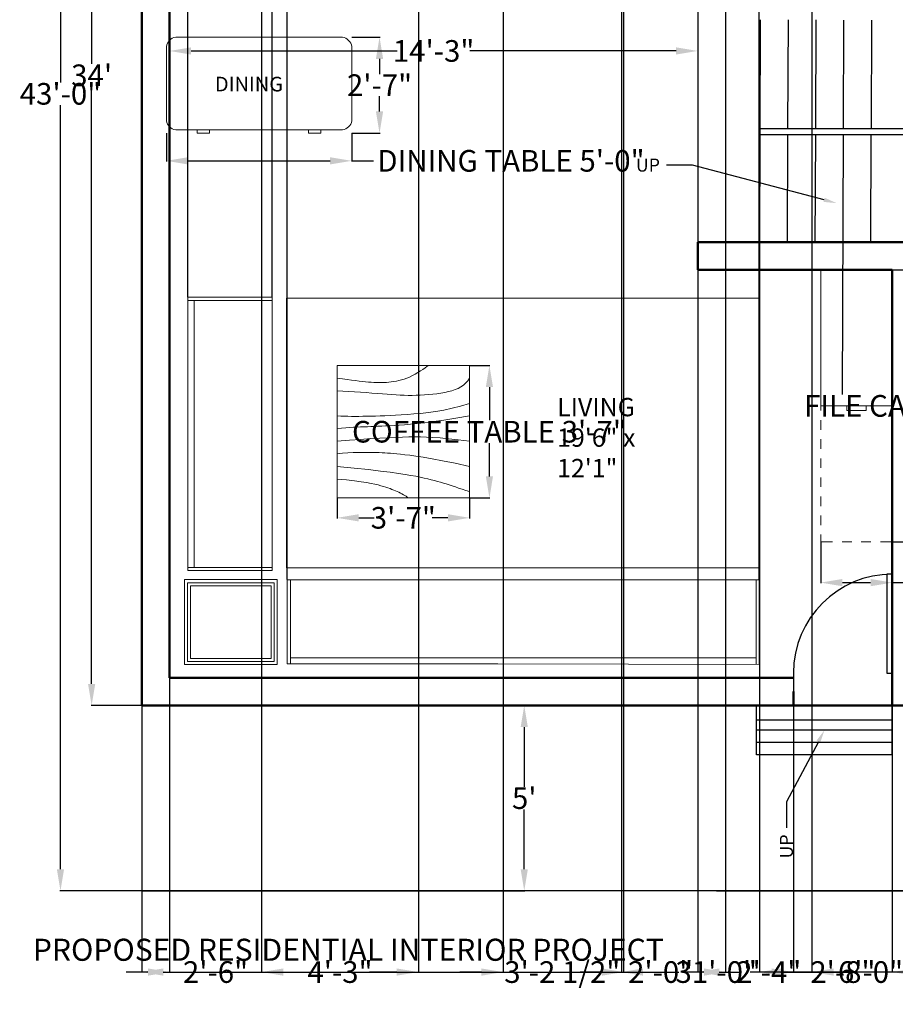
# Model space of a CAD drawing. Units: inches. Extents: x 164 to 612, y 17 to 606.
# Tile 1 of 3: x 164 to 448, y 17 to 335. Entities that reach past the tile are written whole.
import ezdxf
from ezdxf import colors
from ezdxf.entities.mleader import LeaderData, LeaderLine
from ezdxf.math import Vec2, Vec3

# ---------------------------------------------------------------- set-up
doc = ezdxf.new("R2010")
doc.units = ezdxf.units.IN
doc.header["$MEASUREMENT"] = 0
for name, color, linetype, lineweight in [('A-ANNO-DIMS', 2, 'Continuous', 18), ('A-ANNO-TEXT', 7, 'Continuous', 18), ('A-ANNO-TTLB', 7, 'Continuous', 35), ('A-AREA-IDEN', 7, 'Continuous', 25), ('A-DOOR', 4, 'Continuous', 25), ('A-FLOR-STRS', 7, 'Continuous', 25), ('A-FURN', 8, 'Continuous', 18), ('A-WALL', 7, 'Continuous', 50), ('C-PROP', 3, 'Continuous', 25)]:
    doc.layers.add(name, color=color, linetype=linetype, lineweight=lineweight)
doc.styles.get("Standard").update_dxf_attribs({"font": 'arial.ttf'})
doc.dimstyles.get("Standard").update_dxf_attribs({"dimtxt": 7, "dimasz": 7, "dimexe": 0.18, "dimexo": 0.0625, "dimgap": 0.09, "dimtad": 0, "dimtih": 1, "dimtoh": 1, "dimdec": 0, "dimzin": 0, "dimdsep": 46, "dimlunit": 3, "dimtxsty": 'Standard', "dimcen": 0.09, "dimadec": 0, "dimazin": 0, "dimtfac": 1, "dimtdec": 0, "dimtofl": 0, "dimtmove": 0, "dimatfit": 3, "dimfxl": 1, "dimtolj": 1, "dimtzin": 0, "dimarcsym": 0})

# ---------------------------------------------------------------- blocks, each defined once
blk = doc.blocks.new('File Cabinet - Letter')
for p, q in [((0, 0), (15, 0)), ((0, -28.5), (0, 0)), ((15, 0), (15, -28.5)), ((15, -28.5), (0, -28.5)), ((0, -29.5), (0, -28.5)), ((5.5, -28.5), (5.5, -29.5)), ((9.5, -29.5), (9.5, -28.5)), ((5.5, -29.5), (9.5, -29.5)), ((15, -30.5), (15, -32.5)), ((0, -33.5), (0, -31.5)), ((15, -34.5), (15, -36.5)), ((0, -37.5), (0, -35.5)), ((15, -38.5), (15, -40.5)), ((0, -41.5), (0, -39.5)), ((15, -42.5), (15, -44.5)), ((0, -45.5), (0, -43.5)), ((15, -46.5), (15, -48.5)), ((0, -49.5), (0, -47.5)), ((0, -53.5), (0, -51.5)), ((15, -50.5), (15, -52.5)), ((0, -57), (0, -55.5)), ((15, -54.5), (15, -57)), ((2.5, -57), (0, -57)), ((6.5, -57), (4.5, -57)), ((10.5, -57), (8.5, -57)), ((15, -57), (12.5, -57))]:
    blk.add_line(p, q)
blk = doc.blocks.new('Table - Square Woodgrain 42 x 42 in.')
blk.add_line((0, -42), (42, -42))
for points in [[(0, -4), (1.704, -4.2172), (3.2358, -4.4188), (4.615, -4.604), (5.8615, -4.7721), (6.9951, -4.9224), (8.0357, -5.0541), (9.0031, -5.1667), (9.9171, -5.2594), (10.7951, -5.3316), (11.6445, -5.3836), (12.4702, -5.4157), (13.277, -5.4283), (14.0698, -5.4217), (14.8535, -5.3964), (15.6331, -5.3526), (16.4133, -5.2908), (17.1986, -5.2103), (17.9913, -5.1062), (18.793, -4.9727), (19.6056, -4.8038), (20.4307, -4.5937), (21.2701, -4.3365), (22.1256, -4.0262), (22.9989, -3.6571), (23.888, -3.2272), (24.7756, -2.7516), (25.6408, -2.2491), (26.4624, -1.7387), (27.2195, -1.2395), (27.891, -0.7703), (28.456, -0.3501), (28.8934, 0.002)], [(0, -42), (0, 0), (42, 0), (42, -42)], [(0, -8), (1.8203, -8.1001), (3.6741, -8.2149), (5.5411, -8.3408), (7.4011, -8.4741), (9.2339, -8.6112), (11.0193, -8.7484), (12.7371, -8.8821), (14.3671, -9.0086), (15.8954, -9.1246), (17.3337, -9.2278), (18.6997, -9.3159), (20.0116, -9.387), (21.2871, -9.4389), (22.5442, -9.4696), (23.8008, -9.477), (25.0749, -9.459), (26.3791, -9.4137), (27.7049, -9.3403), (29.0383, -9.2382), (30.3655, -9.1068), (31.6728, -8.9455), (32.9461, -8.7535), (34.1717, -8.5304), (35.3358, -8.2756), (36.4268, -7.9863), (37.443, -7.6521), (38.3849, -7.2603), (39.253, -6.7986), (40.048, -6.2542), (40.7705, -5.6147), (41.421, -4.8674), (42, -4)], [(42, -12), (39.1784, -12.8621), (36.4519, -13.5654), (33.8246, -14.1294), (31.3004, -14.5731), (28.8832, -14.9161), (26.577, -15.1775), (24.3858, -15.3768), (22.3136, -15.5332), (20.3622, -15.6632), (18.5254, -15.7718), (16.7947, -15.8612), (15.1618, -15.9338), (13.6183, -15.9916), (12.1558, -16.0369), (10.7659, -16.0718), (9.4403, -16.0987), (8.1703, -16.1191), (6.9461, -16.1325), (5.7577, -16.1377), (4.595, -16.1335), (3.4479, -16.1188), (2.3064, -16.0924), (1.1604, -16.0532), (0, -16)], [(42, -16), (37.6529, -16.7365), (33.8802, -17.329), (30.6179, -17.7961), (27.8015, -18.1561), (25.3668, -18.4275), (23.2497, -18.6288), (21.3859, -18.7785), (19.7111, -18.8949), (18.1693, -18.9939), (16.7375, -19.0795), (15.401, -19.1534), (14.1449, -19.217), (12.9544, -19.2717), (11.8148, -19.3191), (10.7113, -19.3606), (9.6291, -19.3976), (8.5534, -19.4323), (7.47, -19.4689), (6.3643, -19.5122), (5.222, -19.5672), (4.0288, -19.6386), (2.7703, -19.7313), (1.4321, -19.8501), (0, -20)], [(0, -24), (3.9243, -23.6805), (7.4766, -23.4138), (10.6891, -23.1954), (13.5943, -23.0205), (16.2247, -22.8847), (18.6125, -22.7832), (20.7903, -22.7116), (22.7903, -22.6651), (24.6563, -22.642), (26.4764, -22.6507), (28.35, -22.7024), (30.3766, -22.8084), (32.6555, -22.98), (35.2861, -23.2283), (38.3678, -23.5645), (42, -24)], [(42, -32), (37.392, -31.017), (33.4585, -30.2231), (30.1291, -29.5949), (27.3334, -29.109), (25.0009, -28.742), (23.0612, -28.4707), (21.4439, -28.2716), (20.0786, -28.1215), (18.8998, -28.0002), (17.8609, -27.9014), (16.9206, -27.8219), (16.0371, -27.7588), (15.1691, -27.709), (14.2748, -27.6693), (13.3128, -27.6368), (12.2415, -27.6083), (11.0295, -27.5824), (9.6867, -27.5643), (8.233, -27.5608), (6.6884, -27.5787), (5.0728, -27.6248), (3.4062, -27.7058), (1.7086, -27.8286), (0, -28)], [(0, -32), (5.4026, -32.5358), (9.9494, -33.019), (13.7424, -33.4553), (16.8834, -33.8505), (19.4743, -34.2106), (21.6171, -34.5413), (23.4136, -34.8486), (24.9657, -35.1382), (26.3614, -35.4156), (27.6332, -35.6841), (28.7995, -35.9467), (29.8788, -36.2064), (30.8897, -36.4661), (31.8507, -36.7288), (32.7802, -36.9973), (33.6968, -37.2747), (34.6175, -37.5635), (35.5531, -37.8651), (36.5128, -38.1805), (37.506, -38.5108), (38.5421, -38.8568), (39.6302, -39.2197), (40.7797, -39.6004), (42, -40)], [(0, -36), (3.0098, -36.2857), (5.5354, -36.5643), (7.6368, -36.8359), (9.374, -37.1009), (10.807, -37.3597), (11.9957, -37.6126), (13.0002, -37.8599), (13.8804, -38.102), (14.6874, -38.3393), (15.4365, -38.5729), (16.1338, -38.8041), (16.7858, -39.0341), (17.3987, -39.264), (17.9787, -39.4952), (18.5322, -39.7288), (19.0655, -39.9662), (19.5832, -40.2081), (20.0842, -40.4544), (20.5657, -40.7046), (21.0249, -40.9581), (21.459, -41.2144), (21.8653, -41.4731), (22.2409, -41.7335), (22.5831, -41.9951)]]:
    blk.add_lwpolyline(points)
blk = doc.blocks.new('Desk - 30 x 60 in.')
for p, q in [((-26.999995, 0), (26.999995, 0)), ((-29.999995, -27), (-29.999995, -3)), ((29.999995, -3), (29.999995, -27)), ((26.999995, -30), (-26.999995, -30)), ((-20.000005, -30), (-20.000005, -31)), ((-20.000005, -31), (-16.000005, -31)), ((-16.000005, -31), (-16.000005, -30)), ((15.999995, -31), (15.999995, -30)), ((19.999995, -31), (15.999995, -31)), ((19.999995, -30), (19.999995, -31))]:
    blk.add_line(p, q)
for centre, start, end in [((-26.499995, -3.5), 98.1301, 171.8699), ((26.499995, -3.5), 8.130102, 81.8699), ((-26.499995, -26.5), 188.1301, 261.8699), ((26.499995, -26.5), 278.1301, 351.8699)]:
    blk.add_arc(centre, 3.535534, start, end)
blk = doc.blocks.new('*U11')
for p, q in [((0, 0), (0, -6)), ((-32, 0), (-32, -6))]:
    blk.add_line(p, q)
blk.add_lwpolyline([(0, 0), (0, 32), (-1.75, 32), (-1.75, 0)], close=True)
blk.add_arc((0, 0), 32, 90, 180)
blk = doc.blocks.new('*D17')
at = {"layer": 'A-ANNO-DIMS', "color": 0, "lineweight": -2, "transparency": 16777216}
for p, q in [((481.01, 254.38), (468.54, 254.38)), ((468.72, 247.38), (468.72, 157.54)), ((468.72, 60.38), (468.72, 150.22)), ((389.63, 53.38), (468.9, 53.38))]:
    blk.add_line(p, q, dxfattribs=at)
at = {"layer": 'A-ANNO-DIMS', "color": 0, "transparency": 16777216}
for points in [[(467.56, 247.38), (469.89, 247.38), (468.72, 254.38)], [(467.56, 60.38), (469.89, 60.38), (468.72, 53.38)]]:
    blk.add_solid(points, dxfattribs=at)
at = {"layer": 'Defpoints', "color": 0, "transparency": 16777216}
for p in [(481.07, 254.38), (389.57, 53.38), (468.72, 53.38)]:
    blk.add_point(p, dxfattribs=at)
at = {"layer": 'A-ANNO-DIMS', "color": 0, "transparency": 16777216, "insert": (468.72, 153.88), "char_height": 7, "attachment_point": 5}
blk.add_mtext('\\A1;16\'-9"', dxfattribs=at)
blk = doc.blocks.new('*D18')
at = {"layer": 'A-ANNO-DIMS', "color": 0, "lineweight": -2, "transparency": 16777216}
for p, q in [((203.63, 113.38), (327.6, 113.38)), ((327.42, 106.38), (327.42, 87.03)), ((327.42, 60.38), (327.42, 79.73)), ((203.63, 53.38), (327.6, 53.38))]:
    blk.add_line(p, q, dxfattribs=at)
at = {"layer": 'A-ANNO-DIMS', "color": 0, "transparency": 16777216}
for points in [[(326.25, 106.38), (328.59, 106.38), (327.42, 113.38)], [(326.25, 60.38), (328.59, 60.38), (327.42, 53.38)]]:
    blk.add_solid(points, dxfattribs=at)
at = {"layer": 'Defpoints', "color": 0, "transparency": 16777216}
for p in [(203.57, 113.38), (203.57, 53.38), (327.42, 53.38)]:
    blk.add_point(p, dxfattribs=at)
at = {"layer": 'A-ANNO-DIMS', "color": 0, "transparency": 16777216, "insert": (327.42, 83.38), "char_height": 7, "attachment_point": 5}
blk.add_mtext("\\A1;5'", dxfattribs=at)
blk = doc.blocks.new('*D20')
at = {"layer": 'A-ANNO-DIMS', "color": 0, "lineweight": -2, "transparency": 16777216}
for p, q in [((212.57, 401.32), (212.57, 325.08)), ((383.57, 335.32), (383.57, 325.08)), ((219.57, 325.26), (286.29, 325.26)), ((376.57, 325.26), (309.85, 325.26))]:
    blk.add_line(p, q, dxfattribs=at)
at = {"layer": 'A-ANNO-DIMS', "color": 0, "transparency": 16777216}
for points in [[(219.57, 326.42), (219.57, 324.09), (212.57, 325.26)], [(376.57, 326.42), (376.57, 324.09), (383.57, 325.26)]]:
    blk.add_solid(points, dxfattribs=at)
at = {"layer": 'Defpoints', "color": 0, "transparency": 16777216}
for p in [(212.57, 401.38), (383.57, 335.38), (212.57, 325.26)]:
    blk.add_point(p, dxfattribs=at)
at = {"layer": 'A-ANNO-DIMS', "color": 0, "transparency": 16777216, "insert": (298.07, 325.26), "char_height": 7, "attachment_point": 5}
blk.add_mtext('\\A1;14\'-3"', dxfattribs=at)
blk = doc.blocks.new('*D21')
at = {"layer": 'A-ANNO-DIMS', "color": 0, "lineweight": -2, "transparency": 16777216}
for p, q in [((227.33, 521.38), (187.19, 521.38)), ((187.37, 514.38), (187.37, 321.05)), ((187.37, 120.38), (187.37, 313.71)), ((217.32, 113.38), (187.19, 113.38))]:
    blk.add_line(p, q, dxfattribs=at)
at = {"layer": 'A-ANNO-DIMS', "color": 0, "transparency": 16777216}
for points in [[(186.2, 514.38), (188.54, 514.38), (187.37, 521.38)], [(186.2, 120.38), (188.54, 120.38), (187.37, 113.38)]]:
    blk.add_solid(points, dxfattribs=at)
at = {"layer": 'Defpoints', "color": 0, "transparency": 16777216}
for p in [(227.39, 521.38), (187.37, 113.38), (217.38, 113.38)]:
    blk.add_point(p, dxfattribs=at)
at = {"layer": 'A-ANNO-DIMS', "color": 0, "transparency": 16777216, "insert": (187.37, 317.38), "char_height": 7, "attachment_point": 5}
blk.add_mtext("\\A1;34'", dxfattribs=at)
blk = doc.blocks.new('*D30')
at = {"layer": 'A-ANNO-DIMS', "color": 0, "lineweight": -2, "transparency": 16777216}
for p, q in [((446.63, 254.38), (459.95, 254.38)), ((459.77, 247.38), (459.77, 214.08)), ((459.77, 173.36), (459.77, 206.66)), ((446.63, 166.36), (459.95, 166.36))]:
    blk.add_line(p, q, dxfattribs=at)
at = {"layer": 'A-ANNO-DIMS', "color": 0, "transparency": 16777216}
for points in [[(458.61, 247.38), (460.94, 247.38), (459.77, 254.38)], [(458.61, 173.36), (460.94, 173.36), (459.77, 166.36)]]:
    blk.add_solid(points, dxfattribs=at)
at = {"layer": 'Defpoints', "color": 0, "transparency": 16777216}
for p in [(446.57, 254.38), (459.77, 254.38), (446.57, 166.36)]:
    blk.add_point(p, dxfattribs=at)
at = {"layer": 'A-ANNO-DIMS', "color": 0, "transparency": 16777216, "insert": (459.77, 210.37), "char_height": 7, "attachment_point": 5}
blk.add_mtext('\\A1;FILE CABINET 7\'-4"', dxfattribs=at)
blk = doc.blocks.new('*D31')
at = {"layer": 'A-ANNO-DIMS', "color": 0, "lineweight": -2, "transparency": 16777216}
for p, q in [((423.41, 166.29), (423.41, 152.97)), ((446.57, 166.29), (446.57, 152.97)), ((430.41, 153.15), (439.57, 153.15)), ((446.57, 153.15), (453.57, 153.15))]:
    blk.add_line(p, q, dxfattribs=at)
at = {"layer": 'A-ANNO-DIMS', "color": 0, "transparency": 16777216}
for points in [[(430.41, 154.32), (430.41, 151.99), (423.41, 153.15)], [(439.57, 154.32), (439.57, 151.99), (446.57, 153.15)]]:
    blk.add_solid(points, dxfattribs=at)
at = {"layer": 'Defpoints', "color": 0, "transparency": 16777216}
for p in [(423.41, 166.36), (446.57, 166.36), (446.57, 153.15)]:
    blk.add_point(p, dxfattribs=at)
at = {"layer": 'A-ANNO-DIMS', "color": 0, "transparency": 16777216, "insert": (465.35, 153.15), "char_height": 7, "attachment_point": 5}
blk.add_mtext('\\A1;1\'-11"', dxfattribs=at)
blk = doc.blocks.new('*D32')
at = {"layer": 'A-ANNO-DIMS', "color": 0, "lineweight": -2, "transparency": 16777216}
for p, q in [((309.78, 223.44), (316.33, 223.44)), ((316.15, 216.44), (316.15, 205.71)), ((316.15, 187.55), (316.15, 198.28)), ((309.78, 180.55), (316.33, 180.55))]:
    blk.add_line(p, q, dxfattribs=at)
at = {"layer": 'A-ANNO-DIMS', "color": 0, "transparency": 16777216}
for points in [[(314.98, 216.44), (317.31, 216.44), (316.15, 223.44)], [(314.98, 187.55), (317.31, 187.55), (316.15, 180.55)]]:
    blk.add_solid(points, dxfattribs=at)
at = {"layer": 'Defpoints', "color": 0, "transparency": 16777216}
for p in [(309.71, 223.44), (316.15, 223.44), (309.71, 180.55)]:
    blk.add_point(p, dxfattribs=at)
at = {"layer": 'A-ANNO-DIMS', "color": 0, "transparency": 16777216, "insert": (316.15, 202), "char_height": 7, "attachment_point": 5}
blk.add_mtext('\\A1;COFFEE TABLE 3\'-7"', dxfattribs=at)
blk = doc.blocks.new('*D33')
at = {"layer": 'A-ANNO-DIMS', "color": 0, "lineweight": -2, "transparency": 16777216}
for p, q in [((266.82, 180.49), (266.82, 173.94)), ((309.71, 180.49), (309.71, 173.94)), ((273.82, 174.12), (278.88, 174.12)), ((302.71, 174.12), (297.66, 174.12))]:
    blk.add_line(p, q, dxfattribs=at)
at = {"layer": 'A-ANNO-DIMS', "color": 0, "transparency": 16777216}
for points in [[(273.82, 175.29), (273.82, 172.95), (266.82, 174.12)], [(302.71, 175.29), (302.71, 172.95), (309.71, 174.12)]]:
    blk.add_solid(points, dxfattribs=at)
at = {"layer": 'Defpoints', "color": 0, "transparency": 16777216}
for p in [(266.82, 180.55), (309.71, 180.55), (309.71, 174.12)]:
    blk.add_point(p, dxfattribs=at)
at = {"layer": 'A-ANNO-DIMS', "color": 0, "transparency": 16777216, "insert": (288.27, 174.12), "char_height": 7, "attachment_point": 5}
blk.add_mtext('\\A1;3\'-7"', dxfattribs=at)
blk = doc.blocks.new('*D34')
at = {"layer": 'A-ANNO-DIMS', "color": 0, "lineweight": -2, "transparency": 16777216}
for p, q in [((211.57, 298.63), (211.57, 289.51)), ((271.57, 298.63), (271.57, 289.51)), ((218.57, 289.69), (264.57, 289.69)), ((271.57, 289.69), (278.57, 289.69))]:
    blk.add_line(p, q, dxfattribs=at)
at = {"layer": 'A-ANNO-DIMS', "color": 0, "transparency": 16777216}
for points in [[(218.57, 290.86), (218.57, 288.52), (211.57, 289.69)], [(264.57, 290.86), (264.57, 288.52), (271.57, 289.69)]]:
    blk.add_solid(points, dxfattribs=at)
at = {"layer": 'Defpoints', "color": 0, "transparency": 16777216}
for p in [(211.57, 298.69), (271.57, 298.69), (271.57, 289.69)]:
    blk.add_point(p, dxfattribs=at)
at = {"layer": 'A-ANNO-DIMS', "color": 0, "transparency": 16777216, "insert": (323.11, 289.69), "char_height": 7, "attachment_point": 5}
blk.add_mtext('\\A1;DINING TABLE 5\'-0"', dxfattribs=at)
blk = doc.blocks.new('*D35')
at = {"layer": 'A-ANNO-DIMS', "color": 0, "lineweight": -2, "transparency": 16777216}
for p, q in [((271.63, 329.69), (280.75, 329.69)), ((280.57, 322.69), (280.57, 317.79)), ((280.57, 305.69), (280.57, 310.58)), ((271.63, 298.69), (280.75, 298.69))]:
    blk.add_line(p, q, dxfattribs=at)
at = {"layer": 'A-ANNO-DIMS', "color": 0, "transparency": 16777216}
for points in [[(279.4, 322.69), (281.74, 322.69), (280.57, 329.69)], [(279.4, 305.69), (281.74, 305.69), (280.57, 298.69)]]:
    blk.add_solid(points, dxfattribs=at)
at = {"layer": 'Defpoints', "color": 0, "transparency": 16777216}
for p in [(271.57, 329.69), (280.57, 329.69), (271.57, 298.69)]:
    blk.add_point(p, dxfattribs=at)
at = {"layer": 'A-ANNO-DIMS', "color": 0, "transparency": 16777216, "insert": (280.57, 314.19), "char_height": 7, "attachment_point": 5}
blk.add_mtext('\\A1;2\'-7"', dxfattribs=at)
blk = doc.blocks.new('*D42')
at = {"layer": 'A-ANNO-DIMS', "color": 0, "lineweight": -2, "transparency": 16777216}
for p, q in [((203.57, 53.32), (203.57, 26.9)), ((575.57, 53.32), (575.57, 26.9)), ((210.57, 27.08), (377.46, 27.08)), ((568.57, 27.08), (401.68, 27.08))]:
    blk.add_line(p, q, dxfattribs=at)
at = {"layer": 'A-ANNO-DIMS', "color": 0, "transparency": 16777216}
for points in [[(210.57, 28.25), (210.57, 25.91), (203.57, 27.08)], [(568.57, 28.25), (568.57, 25.91), (575.57, 27.08)]]:
    blk.add_solid(points, dxfattribs=at)
at = {"layer": 'Defpoints', "color": 0, "transparency": 16777216}
for p in [(203.57, 53.38), (575.57, 53.38), (575.57, 27.08)]:
    blk.add_point(p, dxfattribs=at)
at = {"layer": 'A-ANNO-DIMS', "color": 0, "transparency": 16777216, "insert": (389.57, 27.08), "char_height": 7, "attachment_point": 5}
blk.add_mtext('\\A1;31\'-0"', dxfattribs=at)
blk = doc.blocks.new('*D43')
at = {"layer": 'A-ANNO-DIMS', "color": 0, "lineweight": -2, "transparency": 16777216}
for p, q in [((203.51, 569.38), (177.09, 569.38)), ((177.27, 562.38), (177.27, 315.05)), ((177.27, 60.38), (177.27, 307.71)), ((203.51, 53.38), (177.09, 53.38))]:
    blk.add_line(p, q, dxfattribs=at)
at = {"layer": 'A-ANNO-DIMS', "color": 0, "transparency": 16777216}
for points in [[(176.1, 562.38), (178.44, 562.38), (177.27, 569.38)], [(176.1, 60.38), (178.44, 60.38), (177.27, 53.38)]]:
    blk.add_solid(points, dxfattribs=at)
at = {"layer": 'Defpoints', "color": 0, "transparency": 16777216}
for p in [(177.27, 569.38), (203.57, 569.38), (203.57, 53.38)]:
    blk.add_point(p, dxfattribs=at)
at = {"layer": 'A-ANNO-DIMS', "color": 0, "transparency": 16777216, "insert": (177.27, 311.38), "char_height": 7, "attachment_point": 5}
blk.add_mtext('\\A1;43\'-0"', dxfattribs=at)
blk = doc.blocks.new('*D48')
at = {"layer": 'A-ANNO-DIMS', "color": 0, "lineweight": -2, "transparency": 16777216}
for p, q in [((414.57, 113.32), (414.57, 26.9)), ((446.57, 113.32), (446.57, 26.9)), ((407.57, 27.08), (400.57, 27.08)), ((453.57, 27.08), (460.57, 27.08))]:
    blk.add_line(p, q, dxfattribs=at)
at = {"layer": 'A-ANNO-DIMS', "color": 0, "transparency": 16777216}
for points in [[(407.57, 28.25), (407.57, 25.91), (414.57, 27.08)], [(453.57, 28.25), (453.57, 25.91), (446.57, 27.08)]]:
    blk.add_solid(points, dxfattribs=at)
at = {"layer": 'Defpoints', "color": 0, "transparency": 16777216}
for p in [(414.57, 113.38), (446.57, 113.38), (446.57, 27.08)]:
    blk.add_point(p, dxfattribs=at)
at = {"layer": 'A-ANNO-DIMS', "color": 0, "transparency": 16777216, "insert": (430.57, 27.08), "char_height": 7, "attachment_point": 5}
blk.add_mtext('\\A1;2\'-8"', dxfattribs=at)
blk = doc.blocks.new('*D49')
at = {"layer": 'A-ANNO-DIMS', "color": 0, "lineweight": -2, "transparency": 16777216}
for p, q in [((392.57, 344.32), (392.57, 26.9)), ((420.57, 344.32), (420.57, 26.9)), ((385.57, 27.08), (378.57, 27.08)), ((427.57, 27.08), (434.57, 27.08))]:
    blk.add_line(p, q, dxfattribs=at)
at = {"layer": 'A-ANNO-DIMS', "color": 0, "transparency": 16777216}
for points in [[(385.57, 28.25), (385.57, 25.91), (392.57, 27.08)], [(427.57, 28.25), (427.57, 25.91), (420.57, 27.08)]]:
    blk.add_solid(points, dxfattribs=at)
at = {"layer": 'Defpoints', "color": 0, "transparency": 16777216}
for p in [(392.57, 344.38), (420.57, 344.38), (420.57, 27.08)]:
    blk.add_point(p, dxfattribs=at)
at = {"layer": 'A-ANNO-DIMS', "color": 0, "transparency": 16777216, "insert": (406.57, 27.08), "char_height": 7, "attachment_point": 5}
blk.add_mtext('\\A1;2\'-4"', dxfattribs=at)
blk = doc.blocks.new('*D50')
at = {"layer": 'A-ANNO-DIMS', "color": 0, "lineweight": -2, "transparency": 16777216}
for p, q in [((359.57, 422.32), (359.57, 26.9)), ((383.57, 422.32), (383.57, 26.9)), ((352.57, 27.08), (345.57, 27.08)), ((390.57, 27.08), (397.57, 27.08))]:
    blk.add_line(p, q, dxfattribs=at)
at = {"layer": 'A-ANNO-DIMS', "color": 0, "transparency": 16777216}
for points in [[(352.57, 28.25), (352.57, 25.91), (359.57, 27.08)], [(390.57, 28.25), (390.57, 25.91), (383.57, 27.08)]]:
    blk.add_solid(points, dxfattribs=at)
at = {"layer": 'Defpoints', "color": 0, "transparency": 16777216}
for p in [(359.57, 422.38), (383.57, 422.38), (383.57, 27.08)]:
    blk.add_point(p, dxfattribs=at)
at = {"layer": 'A-ANNO-DIMS', "color": 0, "transparency": 16777216, "insert": (371.57, 27.08), "char_height": 7, "attachment_point": 5}
blk.add_mtext('\\A1;2\'-0"', dxfattribs=at)
blk = doc.blocks.new('*D52')
at = {"layer": 'A-ANNO-DIMS', "color": 0, "lineweight": -2, "transparency": 16777216}
for p, q in [((403.53, 263.32), (403.53, 26.9)), ((475.53, 263.01), (475.53, 26.9)), ((410.53, 27.08), (430.12, 27.08)), ((468.53, 27.08), (448.95, 27.08))]:
    blk.add_line(p, q, dxfattribs=at)
at = {"layer": 'A-ANNO-DIMS', "color": 0, "transparency": 16777216}
for points in [[(410.53, 28.25), (410.53, 25.91), (403.53, 27.08)], [(468.53, 28.25), (468.53, 25.91), (475.53, 27.08)]]:
    blk.add_solid(points, dxfattribs=at)
at = {"layer": 'Defpoints', "color": 0, "transparency": 16777216}
for p in [(403.53, 263.38), (475.53, 263.08), (475.53, 27.08)]:
    blk.add_point(p, dxfattribs=at)
at = {"layer": 'A-ANNO-DIMS', "color": 0, "transparency": 16777216, "insert": (439.53, 27.08), "char_height": 7, "attachment_point": 5}
blk.add_mtext('\\A1;6\'-0"', dxfattribs=at)
blk = doc.blocks.new('*D54')
at = {"layer": 'A-ANNO-DIMS', "color": 0, "lineweight": -2, "transparency": 16777216}
for p, q in [((212.57, 401.32), (212.57, 26.9)), ((242.38, 401.32), (242.38, 26.9)), ((205.57, 27.08), (198.57, 27.08)), ((249.38, 27.08), (256.38, 27.08))]:
    blk.add_line(p, q, dxfattribs=at)
at = {"layer": 'A-ANNO-DIMS', "color": 0, "transparency": 16777216}
for points in [[(205.57, 28.25), (205.57, 25.91), (212.57, 27.08)], [(249.38, 28.25), (249.38, 25.91), (242.38, 27.08)]]:
    blk.add_solid(points, dxfattribs=at)
at = {"layer": 'Defpoints', "color": 0, "transparency": 16777216}
for p in [(212.57, 401.38), (242.38, 401.38), (242.38, 27.08)]:
    blk.add_point(p, dxfattribs=at)
at = {"layer": 'A-ANNO-DIMS', "color": 0, "transparency": 16777216, "insert": (227.47, 27.08), "char_height": 7, "attachment_point": 5}
blk.add_mtext('\\A1;2\'-6"', dxfattribs=at)
blk = doc.blocks.new('*D55')
at = {"layer": 'A-ANNO-DIMS', "color": 0, "lineweight": -2, "transparency": 16777216}
for p, q in [((242.38, 401.32), (242.38, 26.9)), ((293.15, 401.32), (293.15, 26.9)), ((249.38, 27.08), (258.23, 27.08)), ((286.15, 27.08), (277.3, 27.08))]:
    blk.add_line(p, q, dxfattribs=at)
at = {"layer": 'A-ANNO-DIMS', "color": 0, "transparency": 16777216}
for points in [[(249.38, 28.25), (249.38, 25.91), (242.38, 27.08)], [(286.15, 28.25), (286.15, 25.91), (293.15, 27.08)]]:
    blk.add_solid(points, dxfattribs=at)
at = {"layer": 'Defpoints', "color": 0, "transparency": 16777216}
for p in [(242.38, 401.38), (293.15, 401.38), (293.15, 27.08)]:
    blk.add_point(p, dxfattribs=at)
at = {"layer": 'A-ANNO-DIMS', "color": 0, "transparency": 16777216, "insert": (267.76, 27.08), "char_height": 7, "attachment_point": 5}
blk.add_mtext('\\A1;4\'-3"', dxfattribs=at)
blk = doc.blocks.new('*D56')
at = {"layer": 'A-ANNO-DIMS', "color": 0, "lineweight": -2, "transparency": 16777216}
for p, q in [((250.72, 154.11), (250.72, 595.86)), ((257.72, 595.68), (307.15, 595.68)), ((396.46, 595.68), (347.03, 595.68)), ((403.46, 154.11), (403.46, 595.86))]:
    blk.add_line(p, q, dxfattribs=at)
at = {"layer": 'A-ANNO-DIMS', "color": 0, "transparency": 16777216}
for points in [[(257.72, 596.85), (257.72, 594.51), (250.72, 595.68)], [(396.46, 596.85), (396.46, 594.51), (403.46, 595.68)]]:
    blk.add_solid(points, dxfattribs=at)
at = {"layer": 'Defpoints', "color": 0, "transparency": 16777216}
for p in [(403.46, 595.68), (250.72, 154.05), (403.46, 154.05)]:
    blk.add_point(p, dxfattribs=at)
at = {"layer": 'A-ANNO-DIMS', "color": 0, "transparency": 16777216, "insert": (327.09, 595.68), "char_height": 7, "attachment_point": 5}
blk.add_mtext('\\A1;12\'-8 1/2"', dxfattribs=at)
blk = doc.blocks.new('*D57')
at = {"layer": 'A-ANNO-DIMS', "color": 0, "lineweight": -2, "transparency": 16777216}
for p, q in [((211.55, 595.68), (204.55, 595.68)), ((218.55, 245.57), (218.55, 595.86)), ((245.79, 245.57), (245.79, 595.86)), ((252.79, 595.68), (259.79, 595.68))]:
    blk.add_line(p, q, dxfattribs=at)
at = {"layer": 'A-ANNO-DIMS', "color": 0, "transparency": 16777216}
for points in [[(211.55, 596.85), (211.55, 594.51), (218.55, 595.68)], [(252.79, 596.85), (252.79, 594.51), (245.79, 595.68)]]:
    blk.add_solid(points, dxfattribs=at)
at = {"layer": 'Defpoints', "color": 0, "transparency": 16777216}
for p in [(245.79, 595.68), (218.55, 245.51), (245.79, 245.51)]:
    blk.add_point(p, dxfattribs=at)
at = {"layer": 'A-ANNO-DIMS', "color": 0, "transparency": 16777216, "insert": (232.17, 595.68), "char_height": 7, "attachment_point": 5}
blk.add_mtext('\\A1;2\'-3"', dxfattribs=at)
blk = doc.blocks.new('*D60')
at = {"layer": 'A-ANNO-DIMS', "color": 0, "lineweight": -2, "transparency": 16777216}
for p, q in [((320.57, 365.32), (320.57, 26.9)), ((358.87, 365.32), (358.87, 26.9)), ((313.57, 27.08), (306.57, 27.08)), ((365.87, 27.08), (372.87, 27.08))]:
    blk.add_line(p, q, dxfattribs=at)
at = {"layer": 'A-ANNO-DIMS', "color": 0, "transparency": 16777216}
for points in [[(313.57, 28.25), (313.57, 25.91), (320.57, 27.08)], [(365.87, 28.25), (365.87, 25.91), (358.87, 27.08)]]:
    blk.add_solid(points, dxfattribs=at)
at = {"layer": 'Defpoints', "color": 0, "transparency": 16777216}
for p in [(320.57, 365.38), (358.87, 365.38), (358.87, 27.08)]:
    blk.add_point(p, dxfattribs=at)
at = {"layer": 'A-ANNO-DIMS', "color": 0, "transparency": 16777216, "insert": (339.72, 27.08), "char_height": 7, "attachment_point": 5}
blk.add_mtext('\\A1;3\'-2 1/2"', dxfattribs=at)

msp = doc.modelspace()

# ---------------------------------------------------------------- linework, layer by layer
at = {"layer": 'A-FLOR-STRS'}
for p, q in [((403.83, 335.38), (403.53, 263.38)), ((412.83, 335.34), (412.69, 300.08)), ((421.83, 335.3), (421.69, 300.08)), ((430.83, 335.27), (430.69, 300.08)), ((439.83, 335.23), (439.69, 300.08)), ((475.68, 300.08), (403.68, 300.08)), ((475.68, 298.08), (403.68, 298.08)), ((412.68, 298.08), (412.53, 263.34)), ((421.68, 298.08), (421.53, 263.3)), ((430.68, 298.08), (430.33, 214.04)), ((439.68, 298.08), (439.53, 263.23)), ((446.57, 113.38), (402.65, 113.38)), ((402.65, 97.38), (402.65, 113.38)), ((446.57, 97.38), (446.57, 113.38)), ((446.57, 108.65), (402.65, 108.65)), ((446.57, 105.38), (402.65, 105.38)), ((446.57, 101.38), (402.65, 101.38)), ((446.57, 97.38), (402.65, 97.38))]:
    msp.add_line(p, q, dxfattribs=at)
at = {"layer": 'A-FURN'}
for p, q in [((245.79, 245.51), (218.55, 245.51)), ((218.55, 245.51), (218.55, 225.2)), ((245.79, 225.2), (245.79, 245.51)), ((245.79, 244.51), (218.55, 244.51)), ((220.55, 158.04), (220.55, 244.51)), ((250.49, 225.16), (250.49, 245.23)), ((250.49, 245.23), (403.46, 245.23)), ((403.46, 245.23), (403.46, 225.16)), ((218.55, 157.04), (218.55, 225.2)), ((245.79, 225.2), (245.79, 157.04)), ((403.46, 225.16), (403.46, 157.98)), ((245.79, 158.04), (218.55, 158.04)), ((245.79, 157.04), (218.55, 157.04)), ((403.46, 157.98), (318.88, 157.98)), ((217.38, 126.61), (217.38, 154.13)), ((217.38, 154.13), (247.45, 154.13)), ((218.38, 127.61), (218.38, 153.13)), ((218.38, 153.13), (246.45, 153.13)), ((246.45, 153.13), (246.45, 127.61)), ((247.45, 154.13), (247.45, 126.61)), ((250.72, 126.81), (250.72, 154.05)), ((250.72, 154.05), (318.88, 154.05)), ((251.72, 126.81), (251.72, 154.05)), ((318.88, 154.05), (403.46, 154.05)), ((402.46, 154.05), (402.46, 126.69)), ((403.46, 154.05), (403.46, 126.69)), ((219.38, 152.13), (245.45, 152.13)), ((219.38, 128.61), (219.38, 152.13)), ((245.45, 152.13), (245.45, 128.61)), ((246.45, 127.61), (218.38, 127.61)), ((245.45, 128.61), (219.38, 128.61)), ((317.88, 128.81), (251.72, 128.81)), ((317.88, 128.81), (402.46, 128.81)), ((247.45, 126.61), (217.38, 126.61)), ((318.88, 126.81), (250.72, 126.81)), ((403.46, 126.69), (318.88, 126.81))]:
    msp.add_line(p, q, dxfattribs=at)
msp.add_lwpolyline([(318.88, 157.98), (250.49, 157.98), (250.49, 225.16)], dxfattribs=at)
at = {"layer": 'A-WALL'}
for p, q in [((203.57, 113.38), (203.57, 521.38)), ((212.57, 122.38), (212.57, 401.38)), ((383.57, 254.38), (383.57, 263.38)), ((392.57, 263.38), (383.57, 263.38)), ((392.57, 263.38), (506.57, 263.38)), ((392.57, 254.38), (383.57, 254.38)), ((392.57, 254.38), (446.57, 254.38)), ((446.57, 122.38), (446.57, 254.38)), ((414.57, 122.38), (212.57, 122.38)), ((446.57, 122.38), (446.57, 113.38)), ((414.57, 117.88), (414.57, 113.38)), ((446.57, 113.38), (203.57, 113.38)), ((455.57, 113.38), (446.57, 113.38))]:
    msp.add_line(p, q, dxfattribs=at)
at = {"layer": 'C-PROP'}
for p in [(203.57, 113.38), (575.57, 53.38)]:
    msp.add_line(p, (203.57, 53.38), dxfattribs=at)

# ---------------------------------------------------------------- block references
at = {"layer": 'A-DOOR'}
msp.add_blockref('*U11', (446.57, 123.88), dxfattribs=at)
at = {"layer": 'A-FURN'}
msp.add_blockref('Desk - 30 x 60 in.', (241.57, 329.69), dxfattribs=at)
for name, p, xscale, yscale, zscale in [('File Cabinet - Letter', (423.41, 254.38), 1.5442580192671, 1.5442580192671, 1.5442580192671), ('Table - Square Woodgrain 42 x 42 in.', (266.82, 223.44), 1.021168516251613, 1.021168516251613, 1.021168516251613)]:
    msp.add_blockref(name, p, dxfattribs=dict(at, xscale=xscale, yscale=yscale, zscale=zscale))

# ---------------------------------------------------------------- texts
at = {"layer": 'A-ANNO-TTLB', "insert": (168.34, 37.87), "char_height": 7.1422, "attachment_point": 1}
msp.add_mtext_dynamic_manual_height_columns('PROPOSED RESIDENTIAL INTERIOR PROJECT', width=205.0092, gutter_width=35.71, heights=[0], dxfattribs=at)
at = {"layer": 'A-AREA-IDEN', "attachment_point": 1}
for s, width, gutter_width, insert, char_height in [('DINING ', 783.3472, 23.7, (227.28, 316.9), 4.739), ('LIVING \\P19\'6" x 12\'1"', 44.6054, 29.61, (338.06, 212.93), 5.9228)]:
    msp.add_mtext_dynamic_manual_height_columns(s, width=width, gutter_width=gutter_width, heights=[0], dxfattribs=dict(at, insert=insert, char_height=char_height))

# ---------------------------------------------------------------- dimensions: what is measured, and where the dimension line sits
at = {"layer": 'A-ANNO-DIMS'}
for base, p1, p2, override, picture, middle in [((403.46, 595.68), (250.72, 154.05), (403.46, 154.05), {"dimdec": 1, "dimlfac": 1, "dimrnd": 0, "dimzin": 1, "dimdsep": 46, "dimlunit": 4, "dimfrac": 2}, '*D56', (327.09, 595.68)), ((245.79, 595.68), (218.55, 245.51), (245.79, 245.51), {"dimdec": 1, "dimlfac": 1, "dimrnd": 0, "dimzin": 1, "dimdsep": 46, "dimlunit": 4, "dimfrac": 2}, '*D57', (232.17, 595.68)), ((383.57, 27.08), (359.57, 422.38), (383.57, 422.38), {"dimdec": 1, "dimlfac": 1, "dimrnd": 0, "dimzin": 1, "dimdsep": 46, "dimlunit": 4, "dimfrac": 2}, '*D50', (371.57, 27.08)), ((242.38, 27.08), (212.57, 401.38), (242.38, 401.38), {"dimdec": 1, "dimlfac": 1, "dimrnd": 0, "dimzin": 1, "dimdsep": 46, "dimlunit": 4, "dimfrac": 2}, '*D54', (227.47, 27.08)), ((212.57, 325.26), (383.57, 335.38), (212.57, 401.38), {"dimclrd": 0, "dimclre": 0, "dimclrt": 0}, '*D20', (298.07, 325.26)), ((293.15, 27.08), (242.38, 401.38), (293.15, 401.38), {"dimdec": 1, "dimlfac": 1, "dimrnd": 0, "dimzin": 1, "dimdsep": 46, "dimlunit": 4, "dimfrac": 2}, '*D55', (267.76, 27.08)), ((358.87, 27.08), (320.57, 365.38), (358.87, 365.38), {"dimdec": 1, "dimlfac": 1, "dimrnd": 0, "dimzin": 1, "dimdsep": 46, "dimlunit": 4, "dimfrac": 2}, '*D60', (339.72, 27.08)), ((420.57, 27.08), (392.57, 344.38), (420.57, 344.38), {"dimdec": 1, "dimlfac": 1, "dimrnd": 0, "dimzin": 1, "dimdsep": 46, "dimlunit": 4, "dimfrac": 2}, '*D49', (406.57, 27.08)), ((475.53, 27.08), (403.53, 263.38), (475.53, 263.08), {"dimdec": 1, "dimlfac": 1, "dimrnd": 0, "dimzin": 1, "dimdsep": 46, "dimlunit": 4, "dimfrac": 2}, '*D52', (439.53, 27.08)), ((309.71, 174.12), (266.82, 180.55), (309.71, 180.55), {"dimdec": 1, "dimlfac": 1, "dimrnd": 0, "dimzin": 1, "dimdsep": 46, "dimlunit": 4, "dimfrac": 2}, '*D33', (288.27, 174.12)), ((446.57, 153.15), (423.41, 166.36), (446.57, 166.36), {"dimdec": 1, "dimlfac": 1, "dimrnd": 0, "dimzin": 1, "dimdsep": 46, "dimlunit": 4, "dimfrac": 2}, '*D31', (465.35, 153.15)), ((446.57, 27.08), (414.57, 113.38), (446.57, 113.38), {"dimdec": 1, "dimlfac": 1, "dimrnd": 0, "dimzin": 1, "dimdsep": 46, "dimlunit": 4, "dimfrac": 2}, '*D48', (430.57, 27.08)), ((575.57, 27.08), (203.57, 53.38), (575.57, 53.38), {"dimdec": 1, "dimlfac": 1, "dimrnd": 0, "dimzin": 1, "dimdsep": 46, "dimlunit": 4, "dimfrac": 2}, '*D42', (389.57, 27.08))]:
    dim = msp.add_linear_dim(base=base, p1=p1, p2=p2, dimstyle='Standard', override=override, dxfattribs=at)
    dim.commit()
    dim.dimension.update_dxf_attribs({"geometry": picture, "text_midpoint": middle})
for base, p1, p2, override, picture, middle in [((177.27, 569.38), (203.57, 53.38), (203.57, 569.38), {"dimdec": 1, "dimlfac": 1, "dimrnd": 0, "dimzin": 1, "dimdsep": 46, "dimlunit": 4, "dimfrac": 2}, '*D43', (177.27, 311.38)), ((280.57, 329.69), (271.57, 298.69), (271.57, 329.69), {"dimdec": 1, "dimlfac": 1, "dimrnd": 0, "dimzin": 1, "dimdsep": 46, "dimlunit": 4, "dimfrac": 2}, '*D35', (280.57, 314.19)), ((468.72, 53.38), (481.07, 254.38), (389.57, 53.38), {"dimclrd": 0, "dimclre": 0, "dimclrt": 0}, '*D17', (468.72, 153.88)), ((327.42, 53.38), (203.57, 113.38), (203.57, 53.38), {"dimclrd": 0, "dimclre": 0, "dimclrt": 0}, '*D18', (327.42, 83.38))]:
    dim = msp.add_linear_dim(base=base, p1=p1, p2=p2, angle=90, dimstyle='Standard', override=override, dxfattribs=at)
    dim.commit()
    dim.dimension.update_dxf_attribs({"geometry": picture, "text_midpoint": middle})
dim = msp.add_linear_dim(base=(187.37, 113.38), p1=(227.39, 521.38), p2=(217.38, 113.38), angle=90, dimstyle='Standard', override={"dimclrd": 0, "dimclre": 0, "dimclrt": 0}, dxfattribs=at)
dim.commit()
dim.dimension.update_dxf_attribs({"geometry": '*D21', "text_midpoint": (187.37, 317.38), "dimtype": 160})
dim = msp.add_linear_dim(base=(271.57, 289.69), p1=(211.57, 298.69), p2=(271.57, 298.69), text='DINING TABLE <>', dimstyle='Standard', override={"dimdec": 1, "dimlfac": 1, "dimrnd": 0, "dimzin": 1, "dimdsep": 46, "dimlunit": 4, "dimfrac": 2}, dxfattribs=at)
dim.commit()
dim.dimension.update_dxf_attribs({"geometry": '*D34', "text_midpoint": (323.11, 289.69)})
for base, p1, p2, text, picture, middle in [((459.77, 254.38), (446.57, 166.36), (446.57, 254.38), 'FILE CABINET <>', '*D30', (459.77, 210.37)), ((316.15, 223.44), (309.71, 180.55), (309.71, 223.44), 'COFFEE TABLE <>', '*D32', (316.15, 202))]:
    dim = msp.add_linear_dim(base=base, p1=p1, p2=p2, angle=90, text=text, dimstyle='Standard', override={"dimdec": 1, "dimlfac": 1, "dimrnd": 0, "dimzin": 1, "dimdsep": 46, "dimlunit": 4, "dimfrac": 2}, dxfattribs=at)
    dim.commit()
    dim.dimension.update_dxf_attribs({"geometry": picture, "text_midpoint": middle})

# ---------------------------------------------------------------- leaders
at = {"layer": 'A-ANNO-TEXT'}
ml = msp.add_multileader_mtext('Standard', dxfattribs=at)
ml.set_content('UP', color=256)
ml.set_leader_properties()
ml.build(insert=Vec2(0, 0))
ml.multileader.update_dxf_attribs({"dogleg_length": 0.36, "arrow_head_size": 4.22})
ctx = ml.context
ctx.base_point, ctx.char_height, ctx.arrow_head_size, ctx.landing_gap_size, ctx.plane_origin = Vec3(361.77, 288.28), 4.221, 4.22, 2.11, Vec3(1842.47, 109.42)
ctx.text_align_type = 2
notes = []
notes.append((ctx, [(0, (1, 1, 0), (381.91, 288.28), (-1, 0), 8.44, [(0, [(428.57, 275.99)], 0, [])])]))
ctx.mtext.insert, ctx.mtext.alignment, ctx.mtext.flow_direction = Vec3(371.36, 290.43), 3, 5
ml = msp.add_multileader_mtext('Standard', dxfattribs=at)
ml.set_content('UP', color=256)
ml.set_leader_properties()
ml.build(insert=Vec2(0, 0))
ml.multileader.update_dxf_attribs({"dogleg_length": 0.36, "arrow_head_size": 4.22})
ctx = ml.context
ctx.base_point, ctx.char_height, ctx.arrow_head_size, ctx.landing_gap_size, ctx.plane_origin, ctx.plane_x_axis, ctx.plane_y_axis = Vec3(412.32, 62.07), 4.221, 4.22, 2.11, Vec3(591.17, 1519.28), Vec3(0, 1), Vec3(-1, 0)
ctx.text_align_type = 2
notes.append((ctx, [(0, (1, 1, 0), (412.32, 82.21), (0, -1), 8.44, [(0, [(424.61, 105.38)], 0, [])])]))
ctx.mtext.insert, ctx.mtext.text_direction, ctx.mtext.rotation, ctx.mtext.alignment, ctx.mtext.flow_direction = Vec3(410.17, 71.65), Vec3(0, 1), 1.570796, 3, 5
for ctx, leaders in notes:
    for number, flags, end, landing, length, lines in leaders:
        leader = LeaderData()
        leader.index, (leader.has_last_leader_line, leader.has_dogleg_vector, leader.attachment_direction) = number, flags
        leader.last_leader_point, leader.dogleg_vector, leader.dogleg_length = Vec3(end), Vec3(landing), length
        for number, points, colour, breaks in lines:
            line = LeaderLine()
            line.index, line.vertices, line.color, line.breaks = number, Vec3.list(points), colors.encode_raw_color(colour), breaks
            leader.lines.append(line)
        ctx.leaders.append(leader)

doc.saveas('drawing.dxf')
